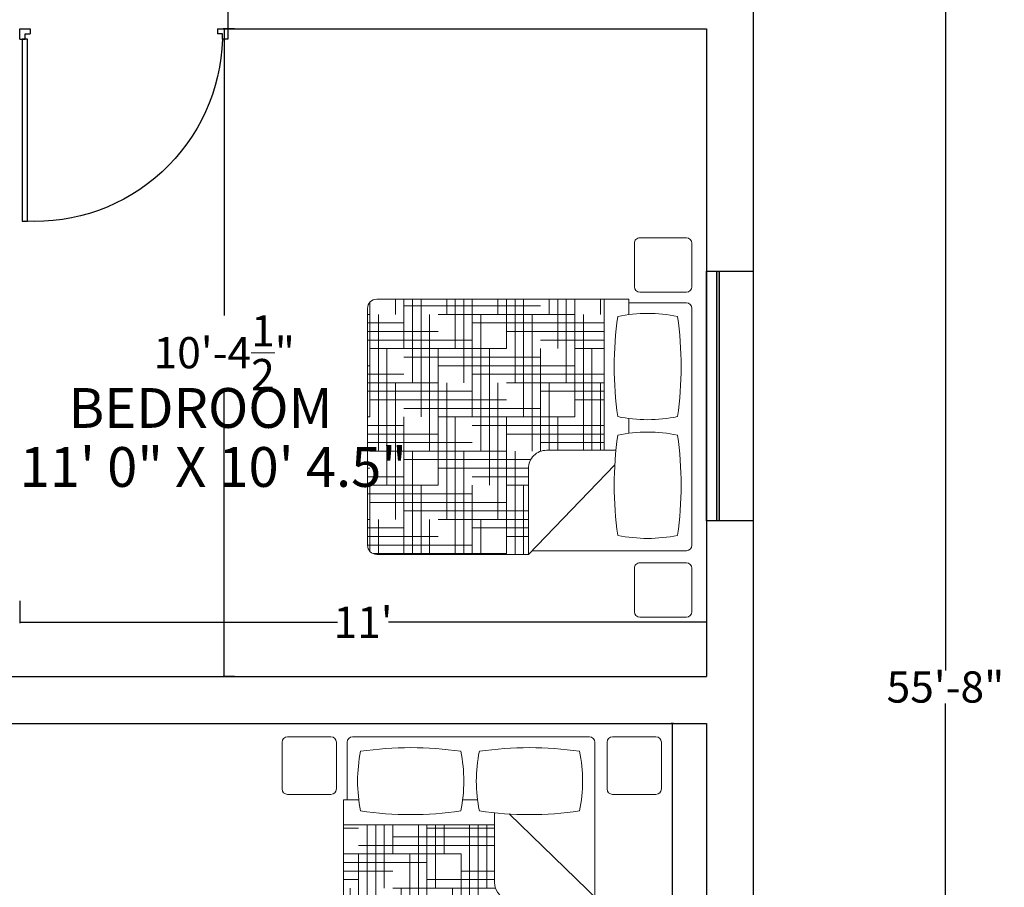
# Model space of a CAD drawing. Units: inches. Extents: x -113 to 5399, y -1393 to 3302.
# Tile 17 of 40: x 1896 to 2086, y 426 to 592. Entities that reach past the tile are written whole.
import ezdxf

# ---------------------------------------------------------------- set-up
doc = ezdxf.new("R2010")
doc.units = ezdxf.units.IN
doc.header["$MEASUREMENT"] = 0
for name, color, linetype, lineweight in [('A-ANNO-DIMS', 254, 'Continuous', 18), ('A-AREA-IDEN', 4, 'Continuous', 18), ('doors', 2, 'Continuous', 25), ('furniture', 131, 'Continuous', 18), ('walls', 1, 'Continuous', 25), ('windows', 3, 'Continuous', 25)]:
    doc.layers.add(name, color=color, linetype=linetype, lineweight=lineweight)
doc.styles.get("Standard").update_dxf_attribs({"font": 'arial.ttf'})
doc.dimstyles.get("Standard").update_dxf_attribs({"dimtxt": 6, "dimasz": 0.18, "dimexe": 0.18, "dimexo": 0.0625, "dimgap": 0.09, "dimtad": 0, "dimtih": 1, "dimtoh": 1, "dimdec": 1, "dimzin": 0, "dimdsep": 46, "dimlunit": 4, "dimtxsty": 'Standard', "dimblk": 'ARCHTICK', "dimcen": 0.09, "dimadec": 0, "dimazin": 0, "dimtfac": 1, "dimtdec": 1, "dimtofl": 0, "dimtmove": 0, "dimatfit": 3, "dimfxl": 1, "dimtolj": 1, "dimtzin": 0, "dimarcsym": 0})

# ---------------------------------------------------------------- blocks, each defined once
blk = doc.blocks.new('*X4')
at = {"color": 0}
for p, q in [((4.3594, 18.5625), (4.3594, 18.6457)), ((4.5, 18), (4.5, 18.6457)), ((4.5469, 18.1875), (4.5469, 18.6457)), ((4.5938, 18.375), (4.5938, 18.6457)), ((4.6406, 18.5625), (4.6406, 18.6457)), ((4.7812, 18), (4.7812, 18.6457)), ((4.8281, 18.1875), (4.8281, 18.6457)), ((4.875, 18.375), (4.875, 18.6457)), ((4.9219, 18.5625), (4.9219, 18.6457)), ((5.0625, 18), (5.0625, 18.6457)), ((5.1094, 18.1875), (5.1094, 18.6457)), ((5.1562, 18.375), (5.1562, 18.6457)), ((5.2031, 18.5625), (5.2031, 18.6457)), ((5.3438, 18), (5.3438, 18.6457)), ((5.3906, 18.1875), (5.3906, 18.6457)), ((5.4375, 18.375), (5.4375, 18.6457)), ((5.4844, 18.5625), (5.4844, 18.6457)), ((4.6875, 18.6094), (5.4375, 18.6094)), ((5.625, 18), (5.625, 18.6287)), ((4.4531, 17.8169), (4.4531, 18.5625)), ((4.5, 18.5625), (5.25, 18.5625)), ((4.7344, 17.8125), (4.7344, 18.5625)), ((5.0156, 17.8125), (5.0156, 18.5625)), ((5.2969, 17.8125), (5.2969, 18.5625)), ((5.5781, 17.8125), (5.5781, 18.5625)), ((5.625, 18.5625), (5.6375, 18.5625)), ((4.3395, 18.5156), (5.0625, 18.5156)), ((5.4375, 18.5156), (5.6375, 18.5156)), ((4.3395, 18.4688), (4.875, 18.4688)), ((5.25, 18.4688), (5.6375, 18.4688)), ((4.3395, 18.4219), (4.6875, 18.4219)), ((4.3395, 18.375), (4.5, 18.375)), ((4.4062, 17.8169), (4.4062, 18.375)), ((4.6875, 17.8114), (4.6875, 18.375)), ((4.875, 18.375), (5.625, 18.375)), ((4.9688, 17.625), (4.9688, 18.375)), ((5.0625, 18.4219), (5.6375, 18.4219)), ((5.25, 17.625), (5.25, 18.375)), ((5.5312, 17.625), (5.5312, 18.375)), ((4.6875, 18.3281), (5.4375, 18.3281)), ((4.5, 18.2812), (5.25, 18.2812)), ((5.625, 18.2812), (5.6375, 18.2812)), ((4.3395, 18.2344), (5.0625, 18.2344)), ((5.4375, 18.2344), (5.6375, 18.2344)), ((4.3395, 18.1875), (4.875, 18.1875)), ((4.3594, 17.8169), (4.3594, 18.1875)), ((4.6406, 17.8169), (4.6406, 18.1875)), ((4.9219, 17.4375), (4.9219, 18.1875)), ((5.2031, 17.4375), (5.2031, 18.1875)), ((5.25, 18.1875), (5.6375, 18.1875)), ((5.4844, 17.4375), (5.4844, 18.1875)), ((4.3395, 18.1406), (4.6875, 18.1406)), ((5.0625, 18.1406), (5.6375, 18.1406)), ((4.3395, 18.0938), (4.5, 18.0938)), ((4.875, 18.0938), (5.625, 18.0938)), ((4.5, 18), (5.25, 18)), ((4.5938, 17.8169), (4.5938, 18)), ((4.6875, 18.0469), (5.4375, 18.0469)), ((4.875, 17.25), (4.875, 18)), ((5.1562, 17.25), (5.1562, 18)), ((5.4375, 17.25), (5.4375, 18)), ((5.625, 18), (5.6375, 18)), ((4.3395, 17.9531), (5.0625, 17.9531)), ((5.4375, 17.9531), (5.6375, 17.9531)), ((4.3395, 17.9062), (4.875, 17.9062)), ((5.25, 17.9062), (5.6375, 17.9062)), ((4.3395, 17.8594), (4.6875, 17.8594)), ((5.0625, 17.8594), (5.6375, 17.8594)), ((4.8281, 17.2457), (4.8281, 17.8125)), ((4.875, 17.8125), (5.625, 17.8125)), ((5.1094, 17.2457), (5.1094, 17.8125)), ((5.3906, 17.2457), (5.3906, 17.8125)), ((4.7421, 17.7656), (5.4375, 17.7656)), ((4.7548, 17.7188), (5.25, 17.7188)), ((4.7548, 17.6719), (5.0625, 17.6719)), ((5.4375, 17.6719), (5.6375, 17.6719)), ((5.625, 17.7188), (5.6375, 17.7188)), ((4.7548, 17.625), (4.875, 17.625)), ((4.7812, 17.2457), (4.7812, 17.625)), ((5.0625, 17.2457), (5.0625, 17.625)), ((5.25, 17.625), (5.6375, 17.625)), ((5.3438, 17.2457), (5.3438, 17.625)), ((5.625, 17.2627), (5.625, 17.625)), ((5.0625, 17.5781), (5.6375, 17.5781)), ((4.875, 17.5312), (5.625, 17.5312)), ((4.7548, 17.4844), (5.4375, 17.4844)), ((4.7548, 17.4375), (5.25, 17.4375)), ((5.0156, 17.2457), (5.0156, 17.4375)), ((5.2969, 17.2457), (5.2969, 17.4375)), ((5.5781, 17.2457), (5.5781, 17.4375)), ((5.625, 17.4375), (5.6375, 17.4375)), ((4.7548, 17.3906), (5.0625, 17.3906)), ((5.4375, 17.3906), (5.6375, 17.3906)), ((4.7548, 17.3438), (4.875, 17.3438)), ((5.0625, 17.2969), (5.6375, 17.2969)), ((5.25, 17.3438), (5.6375, 17.3438)), ((4.875, 17.25), (5.6077, 17.25)), ((4.9688, 17.2457), (4.9688, 17.25)), ((5.25, 17.2457), (5.25, 17.25)), ((5.5312, 17.2457), (5.5312, 17.25))]:
    blk.add_line(p, q, dxfattribs=at)
blk = doc.blocks.new('MAT-P01')
for p, q in [((-0.0213, 0.8164), (-0.0213, 0.5605)), ((0.0087, 0.8464), (0.2471, 0.8464)), ((0.2771, 0.8164), (0.2771, 0.5605)), ((0.3437, 0.8164), (0.3437, -0.0316)), ((0.3737, 0.8464), (1.6737, 0.8464)), ((1.7037, 0.8164), (1.7037, 0.5005)), ((1.7622, 0.8164), (1.7622, 0.5605)), ((1.7922, 0.8464), (2.0306, 0.8464)), ((2.0606, 0.8164), (2.0606, 0.5605)), ((0.0087, 0.5305), (0.2471, 0.5305)), ((0.9879, 0.5005), (1.0693, 0.5005)), ((1.6393, 0.5005), (1.7237, 0.5005)), ((1.7237, 0.5005), (1.7237, -0.8836)), ((1.7922, 0.5305), (2.0306, 0.5305)), ((0.8146, 0.423), (0.3237, -0.0509)), ((0.8949, 0.4293), (0.8949, 0.0491)), ((0.8949, 0.3643), (1.7237, 0.3643)), ((0.8949, 0.3643), (0.8949, 0.0491)), ((0.8949, 0.3643), (1.7237, 0.3643)), ((1.7237, 0.3643), (1.7237, -0.8836)), ((0.3237, -0.0509), (0.7949, -0.0509)), ((0.3237, -0.0509), (0.3237, -0.8836)), ((0.3737, -0.9336), (1.6737, -0.9336))]:
    blk.add_line(p, q)
for centre, radius, start, end in [((0.0087, 0.8164), 0.03, 90, 180), ((0.2471, 0.8164), 0.03, 0, 90), ((0.3737, 0.8164), 0.03, 90, 180), ((1.6737, 0.8164), 0.03, 0, 90), ((1.7922, 0.8164), 0.03, 90, 180), ((2.0306, 0.8164), 0.03, 0, 90), ((1.2251, 0.6034), 0.8138, 168.373, 191.627), ((0.7029, -1.1436), 1.9306, 81.8162, 98.1838), ((0.1806, 0.6034), 0.8138, 348.373, 11.627), ((1.8766, 0.6034), 0.8138, 168.373, 191.627), ((1.3543, -1.1436), 1.9306, 81.8162, 98.1838), ((0.8321, 0.6034), 0.8138, 348.373, 11.627), ((0.0087, 0.5605), 0.03, 180, 270), ((0.2471, 0.5605), 0.03, 270, 0), ((1.7922, 0.5605), 0.03, 180, 270), ((2.0306, 0.5605), 0.03, 270, 0), ((0.7029, 2.3504), 1.9306, 261.8162, 278.1838), ((1.3543, 2.3504), 1.9306, 261.8162, 278.1838), ((0.7949, 0.0491), 0.1, 270, 0), ((0.3737, -0.8836), 0.05, 180, 270), ((1.6737, -0.8836), 0.05, 270, 0)]:
    blk.add_arc(centre, radius, start, end)
at = {"rotation": 270}
blk.add_blockref('*X4', (-16.9221, 4.7038), dxfattribs=at)
blk = doc.blocks.new('_ArchTick')
at = {"color": 0, "linetype": 'ByBlock', "const_width": 0.15}
blk.add_lwpolyline([(-0.5, -0.5), (0.5, 0.5)], dxfattribs=at)
blk = doc.blocks.new('*D63')
at = {"layer": 'A-ANNO-DIMS', "color": 0, "lineweight": -2, "transparency": 16777216}
for p, q in [((2021.95, 457.03), (2021.49, 457.03)), ((2021.67, 457.03), (2021.67, 395.69)), ((2021.67, 328.03), (2021.67, 389.38)), ((2021.95, 328.03), (2021.49, 328.03))]:
    blk.add_line(p, q, dxfattribs=at)
at = {"layer": 'Defpoints', "color": 0, "transparency": 16777216}
for p in [(2022.01, 457.03), (2021.67, 328.03), (2022.01, 328.03)]:
    blk.add_point(p, dxfattribs=at)
at = {"layer": 'A-ANNO-DIMS', "color": 0, "lineweight": -2, "transparency": 16777216, "xscale": 0.18, "yscale": 0.18, "zscale": 0.18}
for p, rotation in [((2021.67, 457.03), 90), ((2021.67, 328.03), 270)]:
    blk.add_blockref('_ArchTick', p, dxfattribs=dict(at, rotation=rotation))
at = {"layer": 'A-ANNO-DIMS', "color": 0, "transparency": 16777216, "insert": (2021.67, 392.53), "char_height": 6, "attachment_point": 5}
blk.add_mtext('\\A1;10\'-9"', dxfattribs=at)
blk = doc.blocks.new('*D81')
at = {"layer": 'A-ANNO-DIMS', "color": 0, "lineweight": -2, "transparency": 16777216}
for p, q in [((1937.54, 590.53), (1935.4, 590.53)), ((1935.58, 590.53), (1935.58, 535.45)), ((1935.58, 466.03), (1935.58, 521.12)), ((1937.54, 466.03), (1935.4, 466.03))]:
    blk.add_line(p, q, dxfattribs=at)
at = {"layer": 'Defpoints', "color": 0, "transparency": 16777216}
for p in [(1937.6, 590.53), (1935.58, 466.03), (1937.6, 466.03)]:
    blk.add_point(p, dxfattribs=at)
at = {"layer": 'A-ANNO-DIMS', "color": 0, "lineweight": -2, "transparency": 16777216, "xscale": 0.18, "yscale": 0.18, "zscale": 0.18}
for p, rotation in [((1935.58, 590.53), 90), ((1935.58, 466.03), 270)]:
    blk.add_blockref('_ArchTick', p, dxfattribs=dict(at, rotation=rotation))
at = {"layer": 'A-ANNO-DIMS', "color": 0, "transparency": 16777216, "insert": (1935.58, 528.28), "char_height": 6, "attachment_point": 5}
blk.add_mtext('\\A1;10\'-4{\\H1x;\\S1/2;}"', dxfattribs=at)
blk = doc.blocks.new('*D82')
at = {"layer": 'A-ANNO-DIMS', "color": 0, "lineweight": -2, "transparency": 16777216}
for p, q in [((1896.26, 480.58), (1896.26, 476.3)), ((2028.26, 480.58), (2028.26, 476.3)), ((1896.26, 476.48), (1957.36, 476.48)), ((2028.26, 476.48), (1967.16, 476.48))]:
    blk.add_line(p, q, dxfattribs=at)
at = {"layer": 'Defpoints', "color": 0, "transparency": 16777216}
for p in [(1896.26, 480.65), (2028.26, 480.65), (2028.26, 476.48)]:
    blk.add_point(p, dxfattribs=at)
at = {"layer": 'A-ANNO-DIMS', "color": 0, "lineweight": -2, "transparency": 16777216, "xscale": 0.18, "yscale": 0.18, "zscale": 0.18, "rotation": 180}
blk.add_blockref('_ArchTick', (1896.26, 476.48), dxfattribs=at)
at = {"layer": 'A-ANNO-DIMS', "color": 0, "lineweight": -2, "transparency": 16777216, "xscale": 0.18, "yscale": 0.18, "zscale": 0.18}
blk.add_blockref('_ArchTick', (2028.26, 476.48), dxfattribs=at)
at = {"layer": 'A-ANNO-DIMS', "color": 0, "transparency": 16777216, "insert": (1962.26, 476.48), "char_height": 6, "attachment_point": 5}
blk.add_mtext("\\A1;11'", dxfattribs=at)
blk = doc.blocks.new('WIN-PLAN-48IN')
h = blk.add_hatch(color=256)
h.dxf.hatch_style = 1
h.paths.add_polyline_path([(48, 2.5), (0, 2.5), (0, 2), (48, 2)])
for p, q in [((0, 9), (48, 9)), ((0, 0), (0, 9)), ((48, 9), (48, 0)), ((48, 2.5), (0, 2.5)), ((48, 2), (0, 2)), ((48, 0), (0, 0))]:
    blk.add_line(p, q)
blk = doc.blocks.new('DOOR-SINGLE-36IN-PLAN')
for p, q in [((0.5, 2), (0.5, 36.98)), ((0.5, 36.98), (1.5, 36.98)), ((1.5, 36.98), (1.5, 2)), ((0, 2), (0, 0)), ((0, 2), (1.04, 2)), ((1.5, 2), (0.5, 2)), ((1.04, 2), (1.04, 0.98)), ((40, 2), (38.96, 2)), ((38.96, 2), (38.96, 0.98)), ((40, 0), (40, 2)), ((1.04, 0.98), (2, 0.98)), ((2, 0), (2, 0.98)), ((38.96, 0.98), (38, 0.98)), ((38, 0), (38, 0.98)), ((0, 0), (2, 0)), ((0, 0), (2, 0)), ((38, 0), (40, 0))]:
    blk.add_line(p, q)
blk.add_arc((2.94, 0.99), 36.04, 1.6003, 93.0893)
blk = doc.blocks.new('*D209')
at = {"layer": 'A-ANNO-DIMS', "color": 0, "lineweight": -2, "transparency": 16777216}
for p, q in [((1754.32, 798.03), (2074.39, 798.03)), ((2074.21, 798.03), (2074.21, 467.19)), ((2074.21, 130.03), (2074.21, 460.88)), ((1754.32, 130.03), (2074.39, 130.03))]:
    blk.add_line(p, q, dxfattribs=at)
at = {"layer": 'Defpoints', "color": 0, "transparency": 16777216}
for p in [(1754.26, 798.03), (2074.21, 798.03), (1754.26, 130.03)]:
    blk.add_point(p, dxfattribs=at)
at = {"layer": 'A-ANNO-DIMS', "color": 0, "lineweight": -2, "transparency": 16777216, "xscale": 0.18, "yscale": 0.18, "zscale": 0.18}
for p, rotation in [((2074.21, 798.03), 90), ((2074.21, 130.03), 270)]:
    blk.add_blockref('_ArchTick', p, dxfattribs=dict(at, rotation=rotation))
at = {"layer": 'A-ANNO-DIMS', "color": 0, "transparency": 16777216, "insert": (2074.21, 464.03), "char_height": 6, "attachment_point": 5}
blk.add_mtext('\\A1;55\'-8"', dxfattribs=at)

msp = doc.modelspace()

# ---------------------------------------------------------------- linework, layer by layer
at = {"layer": 'walls'}
for p, q in [((2037.26, 786.53), (2037.26, 136.53)), ((1936.26, 619.53), (1936.26, 590.53)), ((1936.26, 590.53), (2028.26, 590.53)), ((2028.26, 590.53), (2028.26, 466.03)), ((1879.26, 466.03), (2028.26, 466.03)), ((1879.26, 457.03), (2028.26, 457.03)), ((2028.26, 457.03), (2028.26, 332.53))]:
    msp.add_line(p, q, dxfattribs=at)

# ---------------------------------------------------------------- block references
at = {"layer": 'doors', "extrusion": (0, 0, -1), "zscale": -1, "rotation": 180}
msp.add_blockref('DOOR-SINGLE-36IN-PLAN', (-1896.26, 590.53), dxfattribs=at)
at = {"layer": 'furniture', "xscale": -35.02364872074636, "yscale": 35.02364872074636, "zscale": 35.02364872074636, "rotation": 270}
msp.add_blockref('MAT-P01', (1995.83, 478.19), dxfattribs=at)
at = {"layer": 'furniture', "xscale": -35.02364872074636, "yscale": 35.02364872074636, "zscale": 35.02364872074636}
msp.add_blockref('MAT-P01', (2018.86, 424.81), dxfattribs=at)
at = {"layer": 'windows', "rotation": 269.9999999999995}
msp.add_blockref('WIN-PLAN-48IN', (2028.26, 543.95), dxfattribs=at)

# ---------------------------------------------------------------- texts
at = {"layer": 'A-AREA-IDEN'}
for s, height, p in [('BEDROOM', 7.647, (1905.66, 513.84)), ('11\' 0" X 10\' 4.5"', 7.6473, (1896.26, 502.5))]:
    msp.add_text(s, height=height, dxfattribs=at).set_placement(p)

# ---------------------------------------------------------------- dimensions: what is measured, and where the dimension line sits
at = {"layer": 'A-ANNO-DIMS'}
for base, p1, p2, override, picture, middle in [((2074.21, 798.03), (1754.26, 130.03), (1754.26, 798.03), {"dimdec": 1, "dimlfac": 1, "dimrnd": 0, "dimzin": 1, "dimdsep": 46, "dimlunit": 4, "dimfrac": 2}, '*D209', (2074.21, 464.03)), ((1935.58, 466.03), (1937.6, 590.53), (1937.6, 466.03), {"dimclrd": 0, "dimclre": 0, "dimclrt": 0}, '*D81', (1935.58, 528.28)), ((2021.67, 328.03), (2022.01, 457.03), (2022.01, 328.03), {"dimclrd": 0, "dimclre": 0, "dimclrt": 0}, '*D63', (2021.67, 392.53))]:
    dim = msp.add_linear_dim(base=base, p1=p1, p2=p2, angle=90, dimstyle='Standard', override=override, dxfattribs=at)
    dim.commit()
    dim.dimension.update_dxf_attribs({"geometry": picture, "text_midpoint": middle})
dim = msp.add_linear_dim(base=(2028.26, 476.48), p1=(1896.26, 480.65), p2=(2028.26, 480.65), dimstyle='Standard', override={"dimclrd": 0, "dimclre": 0, "dimclrt": 0}, dxfattribs=at)
dim.commit()
dim.dimension.update_dxf_attribs({"geometry": '*D82', "text_midpoint": (1962.26, 476.48)})

doc.saveas('drawing.dxf')
